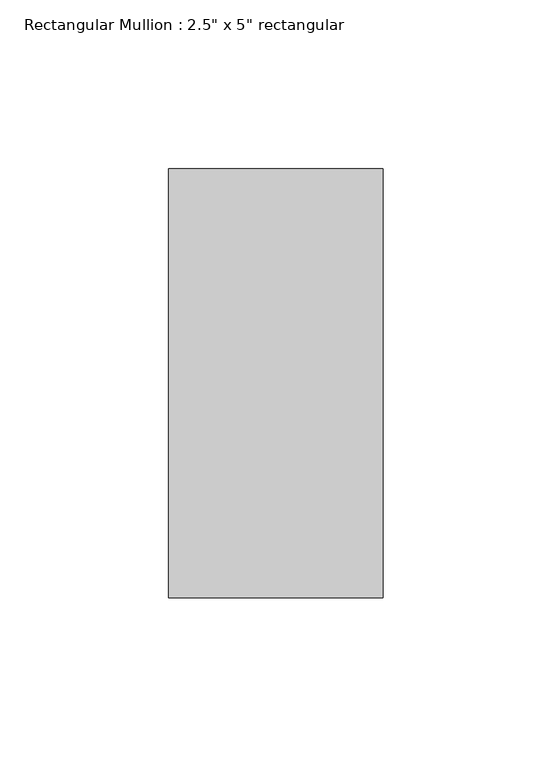
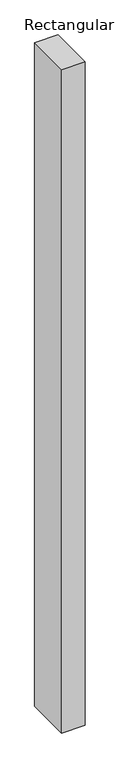
"""IFC4 building model written with IfcOpenShell, lengths in millimetres: member geometry."""

from ifc_helpers import new_model, si_unit, frame, origin, place, context, project, spatial, polyline, outline, extrude, source, transform, mapped, element, save


def member_11fc1043(model_context):
    return source(origin(), model_context, "Body", "SweptSolid", [
        extrude(outline(polyline([(0.0, 63.5), (0.0, -63.5), (-63.5, -63.5), (-63.5, 63.5), (0.0, 63.5)])), frame((0.0, 0.0, -1902.8833333), z_axis=(0.0, 0.0, 1.0), x_axis=(1.0, 0.0, 0.0)), (0.0, 0.0, 1.0), 1902.8833333),
    ])


if __name__ == "__main__":
    model = new_model("IFC4")
    model_context = context("Model", 3, world=origin())
    ifc_project = project(units=[si_unit("LENGTHUNIT", "METRE", prefix="MILLI")], contexts=[model_context])
    site = spatial("IfcSite", under=ifc_project)
    building = spatial("IfcBuilding", under=site)
    placement = place(None, origin())
    member_shape = member_11fc1043(model_context)
    element("IfcMember", 1, ObjectType="Rectangular Mullion : 2.5\" x 5\" rectangular", at=placement, inside=building, context=model_context, shape_type="MappedRepresentation", body=[
        mapped(member_shape, transform((0.0, 0.0, 0.0), x_axis=(1.0, 0.0, 0.0), y_axis=(0.0, 1.0, 0.0), z_axis=(0.0, 0.0, 1.0))),
    ])
    save(model, "model.ifc")

# Revit data of these elements
# Type "Rectangular Mullion : 2.5\" x 5\" rectangular"
#   built-in parameter 1007304 = 0.416667 (stored number, unit not read)
#   built-in parameter 1007301 = 0.104167 (stored number, unit not read)
#   built-in parameter 1007300 = 0.104167 (stored number, unit not read)
# Element 1 (IfcMember, "Rectangular Mullion : 2.5\" x 5\" rectangular")
#   Materials on its faces: "Aluminum"
# Materials
#   "Aluminum": class "Metal", colour RGB 247 247 247, transparency 0, Description = "Aluminum 6061", Cost = 0
